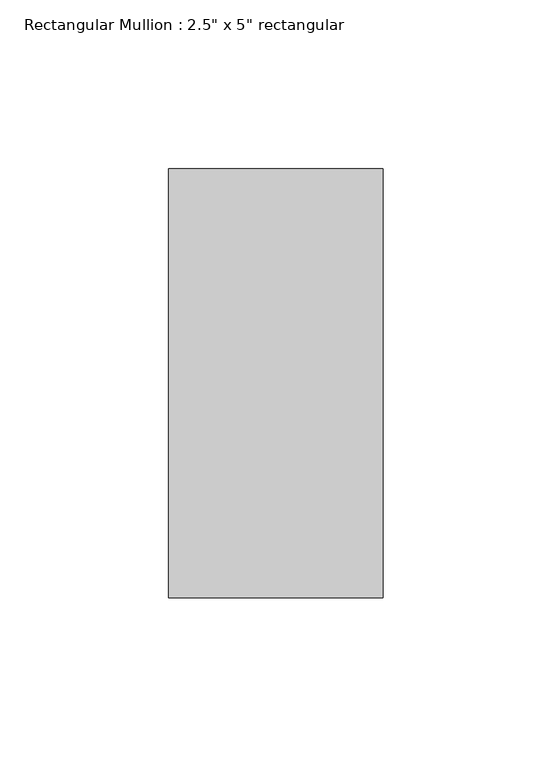
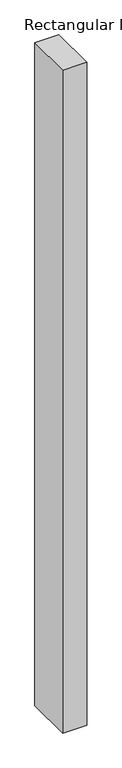
"""IFC4 building model written with IfcOpenShell, lengths in millimetres: member geometry."""

from ifc_helpers import new_model, si_unit, frame, origin, place, context, project, spatial, polyline, outline, extrude, source, transform, mapped, element, save


def member_bdc0ab2a(model_context):
    return source(origin(), model_context, "Body", "SweptSolid", [
        extrude(outline(polyline([(0.0, 63.5), (0.0, -63.5), (-63.5, -63.5), (-63.5, 63.5), (0.0, 63.5)])), frame((0.0, 0.0, -1854.2), z_axis=(0.0, 0.0, 1.0), x_axis=(1.0, 0.0, 0.0)), (0.0, 0.0, 1.0), 1854.2),
    ])


if __name__ == "__main__":
    model = new_model("IFC4")
    model_context = context("Model", 3, world=origin())
    ifc_project = project(units=[si_unit("LENGTHUNIT", "METRE", prefix="MILLI")], contexts=[model_context])
    site = spatial("IfcSite", under=ifc_project)
    building = spatial("IfcBuilding", under=site)
    placement = place(None, origin())
    member_shape = member_bdc0ab2a(model_context)
    element("IfcMember", 1, ObjectType="Rectangular Mullion : 2.5\" x 5\" rectangular", at=placement, inside=building, context=model_context, shape_type="MappedRepresentation", body=[
        mapped(member_shape, transform((0.0, 0.0, 0.0), x_axis=(1.0, 0.0, 0.0), y_axis=(0.0, 1.0, 0.0), z_axis=(0.0, 0.0, 1.0))),
    ])
    save(model, "model.ifc")

# Revit data of these elements
# Type "Rectangular Mullion : 2.5\" x 5\" rectangular"
#   built-in parameter 1007304 = 0.416667 (stored number, unit not read)
#   built-in parameter 1007301 = 0.104167 (stored number, unit not read)
#   built-in parameter 1007300 = 0.104167 (stored number, unit not read)
# Element 1 (IfcMember, "Rectangular Mullion : 2.5\" x 5\" rectangular")
#   Materials on its faces: "Aluminum"
# Materials
#   "Aluminum": class "Metal", colour RGB 247 247 247, transparency 0, Description = "Aluminum 6061", Cost = 0
